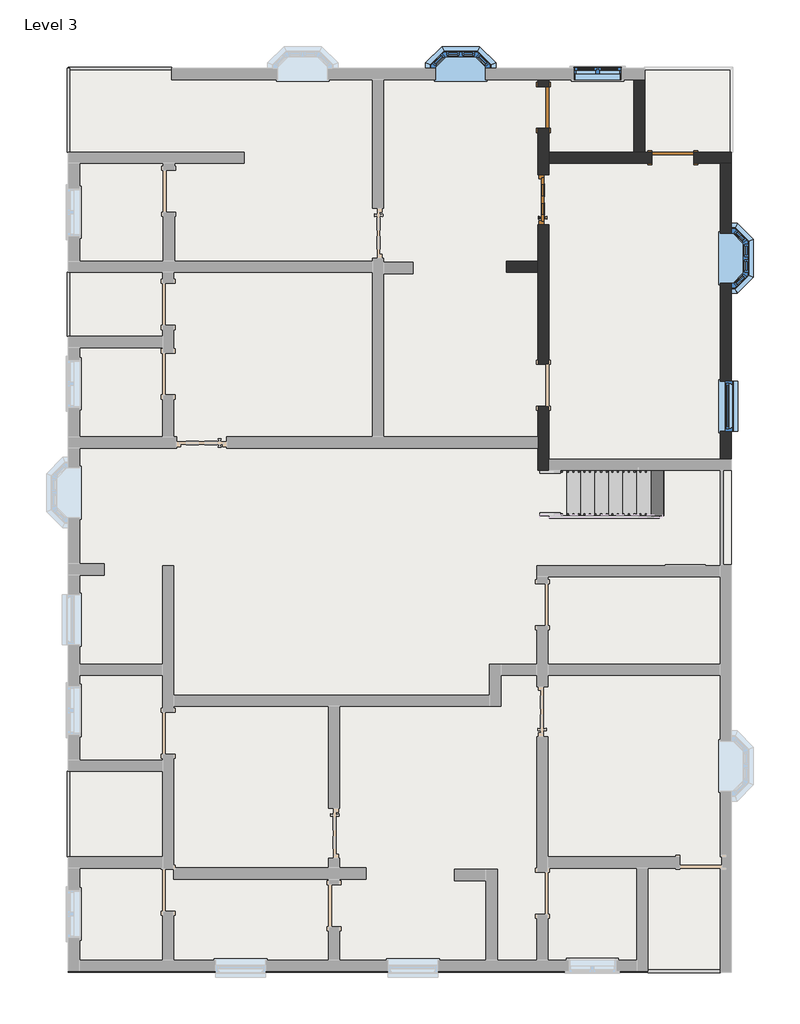
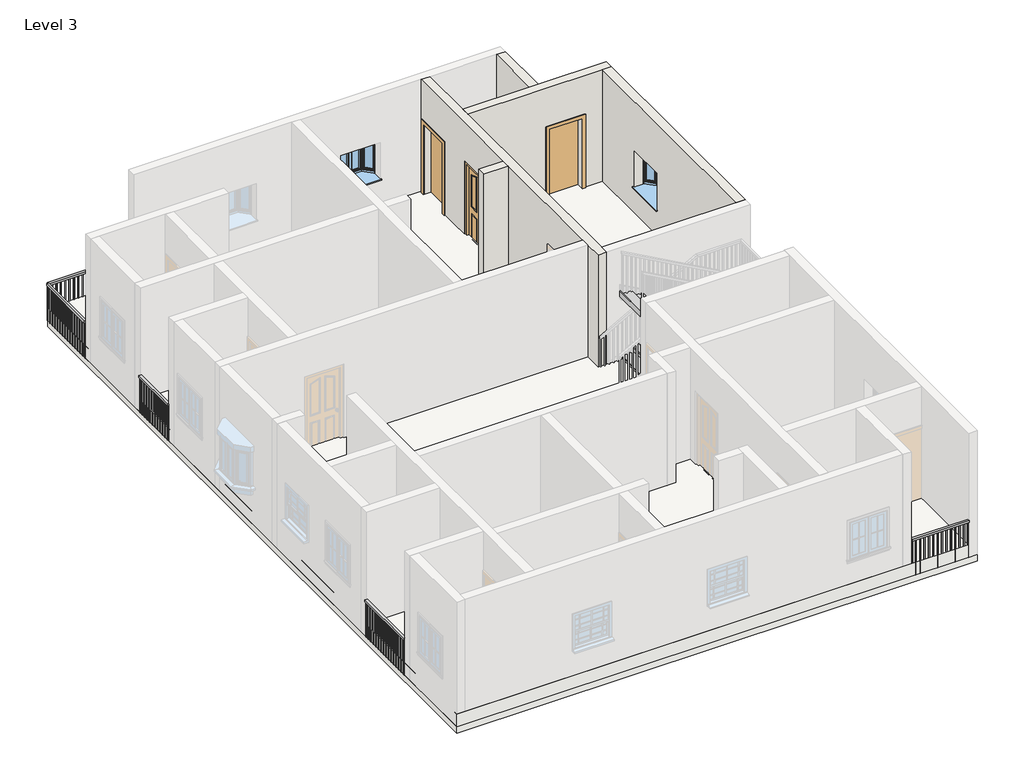
# One storey, part 2 of 4: 5 railings, 5 walls, 4 windows, 3 doors, 1 roof, 1 slab, 1 stair flight.
"""IFC4 building model written with IfcOpenShell, lengths in millimetres."""

from ifc_helpers import new_model, si_unit, frame, origin, place, context, project, spatial, polyline, outline, extrude, faceted_brep, transform, mapped, element, save
from components import doors_extsgl_12_910x2110mm_9a09825e, door_53b1b562, stair_flight_3990532a, window_910x910mm_67ef725a, window_c29befe5, windows_sash_w_bars_1_910x910mm_b688f793

model = new_model("IFC4")

# Units and contexts
model_context = context("Model", 3, world=origin())
ifc_project = project(units=[si_unit("LENGTHUNIT", "METRE", prefix="MILLI")], contexts=[model_context])

# Site, building, storey
site = spatial("IfcSite", under=ifc_project)
building = spatial("IfcBuilding", under=site)
storey = spatial("IfcBuildingStorey", under=building, Name="Level 3", Elevation=6096.0)

# Doors
placement = place(None, origin())
doors_extsgl_12_910x2110mm_shape = doors_extsgl_12_910x2110mm_9a09825e(model_context)
element("IfcDoor", 1, ObjectType="Doors_ExtSgl_12 : 910x2110mm", at=placement, inside=storey, context=model_context, shape_type="MappedRepresentation", body=[
    mapped(doors_extsgl_12_910x2110mm_shape, transform((1600.6941283, 5934.0547293, 6096.0), x_axis=(0.0, 1.0, 0.0), y_axis=(-1.0, 0.0, 0.0), z_axis=(0.0, 0.0, 1.0))),
])
door_shape = door_53b1b562(model_context)
element("IfcDoor", 2, ObjectType="Single-Flush : 30\" x 80\"", at=placement, inside=storey, context=model_context, shape_type="MappedRepresentation", body=[
    mapped(door_shape, transform((1600.6941283, 7610.4547293, 6096.0), x_axis=(0.0, 1.0, 0.0), y_axis=(-1.0, 0.0, 0.0), z_axis=(0.0, 0.0, 1.0))),
])
element("IfcDoor", 3, ObjectType="Single-Flush : 30\" x 80\"", at=placement, inside=storey, context=model_context, shape_type="MappedRepresentation", body=[
    mapped(door_shape, transform((3962.8941283, 6696.0547293, 6096.0), x_axis=(-1.0, 0.0, 0.0), y_axis=(0.0, -1.0, 0.0), z_axis=(0.0, 0.0, 1.0))),
])

# Railings
element("IfcRailing", 4, ObjectType="Handrail - Rectangular", at=placement, inside=storey, context=model_context, shape_type="SweptSolid", body=[
    extrude(outline(polyline([(-7073.4058717, 4609.0339901), (-7022.6058717, 4609.0339901), (-7022.6058717, 3444.8547293), (-7073.4058717, 3444.8547293), (-7073.4058717, 4609.0339901)])), frame((0.0, 0.0, 6959.6), z_axis=(0.0, 0.0, 1.0), x_axis=(1.0, 0.0, 0.0)), (0.0, 0.0, 1.0), 50.8),
    extrude(outline(polyline([(-7057.5308717, 3500.9589901), (-7038.4808717, 3500.9589901), (-7038.4808717, 3481.9089901), (-7057.5308717, 3481.9089901), (-7057.5308717, 3500.9589901)])), frame((0.0, 0.0, 6096.0), z_axis=(0.0, 0.0, 1.0), x_axis=(1.0, 0.0, 0.0)), (0.0, 0.0, 1.0), 863.6),
    extrude(outline(polyline([(-7057.5308717, 3602.5589901), (-7038.4808717, 3602.5589901), (-7038.4808717, 3583.5089901), (-7057.5308717, 3583.5089901), (-7057.5308717, 3602.5589901)])), frame((0.0, 0.0, 6096.0), z_axis=(0.0, 0.0, 1.0), x_axis=(1.0, 0.0, 0.0)), (0.0, 0.0, 1.0), 863.6),
    extrude(outline(polyline([(-7057.5308717, 3704.1589901), (-7038.4808717, 3704.1589901), (-7038.4808717, 3685.1089901), (-7057.5308717, 3685.1089901), (-7057.5308717, 3704.1589901)])), frame((0.0, 0.0, 6096.0), z_axis=(0.0, 0.0, 1.0), x_axis=(1.0, 0.0, 0.0)), (0.0, 0.0, 1.0), 863.6),
    extrude(outline(polyline([(-7057.5308717, 3805.7589901), (-7038.4808717, 3805.7589901), (-7038.4808717, 3786.7089901), (-7057.5308717, 3786.7089901), (-7057.5308717, 3805.7589901)])), frame((0.0, 0.0, 6096.0), z_axis=(0.0, 0.0, 1.0), x_axis=(1.0, 0.0, 0.0)), (0.0, 0.0, 1.0), 863.6),
    extrude(outline(polyline([(-7057.5308717, 3907.3589901), (-7038.4808717, 3907.3589901), (-7038.4808717, 3888.3089901), (-7057.5308717, 3888.3089901), (-7057.5308717, 3907.3589901)])), frame((0.0, 0.0, 6096.0), z_axis=(0.0, 0.0, 1.0), x_axis=(1.0, 0.0, 0.0)), (0.0, 0.0, 1.0), 863.6),
    extrude(outline(polyline([(-7057.5308717, 4008.9589901), (-7038.4808717, 4008.9589901), (-7038.4808717, 3989.9089901), (-7057.5308717, 3989.9089901), (-7057.5308717, 4008.9589901)])), frame((0.0, 0.0, 6096.0), z_axis=(0.0, 0.0, 1.0), x_axis=(1.0, 0.0, 0.0)), (0.0, 0.0, 1.0), 863.6),
    extrude(outline(polyline([(-7057.5308717, 4110.5589901), (-7038.4808717, 4110.5589901), (-7038.4808717, 4091.5089901), (-7057.5308717, 4091.5089901), (-7057.5308717, 4110.5589901)])), frame((0.0, 0.0, 6096.0), z_axis=(0.0, 0.0, 1.0), x_axis=(1.0, 0.0, 0.0)), (0.0, 0.0, 1.0), 863.6),
    extrude(outline(polyline([(-7057.5308717, 4212.1589901), (-7038.4808717, 4212.1589901), (-7038.4808717, 4193.1089901), (-7057.5308717, 4193.1089901), (-7057.5308717, 4212.1589901)])), frame((0.0, 0.0, 6096.0), z_axis=(0.0, 0.0, 1.0), x_axis=(1.0, 0.0, 0.0)), (0.0, 0.0, 1.0), 863.6),
    extrude(outline(polyline([(-7057.5308717, 4313.7589901), (-7038.4808717, 4313.7589901), (-7038.4808717, 4294.7089901), (-7057.5308717, 4294.7089901), (-7057.5308717, 4313.7589901)])), frame((0.0, 0.0, 6096.0), z_axis=(0.0, 0.0, 1.0), x_axis=(1.0, 0.0, 0.0)), (0.0, 0.0, 1.0), 863.6),
    extrude(outline(polyline([(-7057.5308717, 4415.3589901), (-7038.4808717, 4415.3589901), (-7038.4808717, 4396.3089901), (-7057.5308717, 4396.3089901), (-7057.5308717, 4415.3589901)])), frame((0.0, 0.0, 6096.0), z_axis=(0.0, 0.0, 1.0), x_axis=(1.0, 0.0, 0.0)), (0.0, 0.0, 1.0), 863.6),
    extrude(outline(polyline([(-7057.5308717, 4516.9589901), (-7038.4808717, 4516.9589901), (-7038.4808717, 4497.9089901), (-7057.5308717, 4497.9089901), (-7057.5308717, 4516.9589901)])), frame((0.0, 0.0, 6096.0), z_axis=(0.0, 0.0, 1.0), x_axis=(1.0, 0.0, 0.0)), (0.0, 0.0, 1.0), 863.6),
    extrude(outline(polyline([(-7057.5308717, 3463.9047293), (-7038.4808717, 3463.9047293), (-7038.4808717, 3444.8547293), (-7057.5308717, 3444.8547293), (-7057.5308717, 3463.9047293)])), frame((0.0, 0.0, 6096.0), z_axis=(0.0, 0.0, 1.0), x_axis=(1.0, 0.0, 0.0)), (0.0, 0.0, 1.0), 863.6),
    extrude(outline(polyline([(-7057.5308717, 4609.0339901), (-7038.4808717, 4609.0339901), (-7038.4808717, 4589.9839901), (-7057.5308717, 4589.9839901), (-7057.5308717, 4609.0339901)])), frame((0.0, 0.0, 6096.0), z_axis=(0.0, 0.0, 1.0), x_axis=(1.0, 0.0, 0.0)), (0.0, 0.0, 1.0), 863.6),
])
element("IfcRailing", 5, ObjectType="Handrail - Rectangular", at=placement, inside=storey, context=model_context, shape_type="SweptSolid", body=[
    extrude(outline(polyline([(-7073.4058717, -4474.6886333), (-7022.6058717, -4474.6886333), (-7022.6058717, -6029.3452707), (-7073.4058717, -6029.3452707), (-7073.4058717, -4474.6886333)])), frame((0.0, 0.0, 6959.6), z_axis=(0.0, 0.0, 1.0), x_axis=(1.0, 0.0, 0.0)), (0.0, 0.0, 1.0), 50.8),
    extrude(outline(polyline([(-7057.5308717, -5989.1636333), (-7038.4808717, -5989.1636333), (-7038.4808717, -6008.2136333), (-7057.5308717, -6008.2136333), (-7057.5308717, -5989.1636333)])), frame((0.0, 0.0, 6096.0), z_axis=(0.0, 0.0, 1.0), x_axis=(1.0, 0.0, 0.0)), (0.0, 0.0, 1.0), 863.6),
    extrude(outline(polyline([(-7057.5308717, -5887.5636333), (-7038.4808717, -5887.5636333), (-7038.4808717, -5906.6136333), (-7057.5308717, -5906.6136333), (-7057.5308717, -5887.5636333)])), frame((0.0, 0.0, 6096.0), z_axis=(0.0, 0.0, 1.0), x_axis=(1.0, 0.0, 0.0)), (0.0, 0.0, 1.0), 863.6),
    extrude(outline(polyline([(-7057.5308717, -5785.9636333), (-7038.4808717, -5785.9636333), (-7038.4808717, -5805.0136333), (-7057.5308717, -5805.0136333), (-7057.5308717, -5785.9636333)])), frame((0.0, 0.0, 6096.0), z_axis=(0.0, 0.0, 1.0), x_axis=(1.0, 0.0, 0.0)), (0.0, 0.0, 1.0), 863.6),
    extrude(outline(polyline([(-7057.5308717, -5684.3636333), (-7038.4808717, -5684.3636333), (-7038.4808717, -5703.4136333), (-7057.5308717, -5703.4136333), (-7057.5308717, -5684.3636333)])), frame((0.0, 0.0, 6096.0), z_axis=(0.0, 0.0, 1.0), x_axis=(1.0, 0.0, 0.0)), (0.0, 0.0, 1.0), 863.6),
    extrude(outline(polyline([(-7057.5308717, -5582.7636333), (-7038.4808717, -5582.7636333), (-7038.4808717, -5601.8136333), (-7057.5308717, -5601.8136333), (-7057.5308717, -5582.7636333)])), frame((0.0, 0.0, 6096.0), z_axis=(0.0, 0.0, 1.0), x_axis=(1.0, 0.0, 0.0)), (0.0, 0.0, 1.0), 863.6),
    extrude(outline(polyline([(-7057.5308717, -5481.1636333), (-7038.4808717, -5481.1636333), (-7038.4808717, -5500.2136333), (-7057.5308717, -5500.2136333), (-7057.5308717, -5481.1636333)])), frame((0.0, 0.0, 6096.0), z_axis=(0.0, 0.0, 1.0), x_axis=(1.0, 0.0, 0.0)), (0.0, 0.0, 1.0), 863.6),
    extrude(outline(polyline([(-7057.5308717, -5379.5636333), (-7038.4808717, -5379.5636333), (-7038.4808717, -5398.6136333), (-7057.5308717, -5398.6136333), (-7057.5308717, -5379.5636333)])), frame((0.0, 0.0, 6096.0), z_axis=(0.0, 0.0, 1.0), x_axis=(1.0, 0.0, 0.0)), (0.0, 0.0, 1.0), 863.6),
    extrude(outline(polyline([(-7057.5308717, -5277.9636333), (-7038.4808717, -5277.9636333), (-7038.4808717, -5297.0136333), (-7057.5308717, -5297.0136333), (-7057.5308717, -5277.9636333)])), frame((0.0, 0.0, 6096.0), z_axis=(0.0, 0.0, 1.0), x_axis=(1.0, 0.0, 0.0)), (0.0, 0.0, 1.0), 863.6),
    extrude(outline(polyline([(-7057.5308717, -5176.3636333), (-7038.4808717, -5176.3636333), (-7038.4808717, -5195.4136333), (-7057.5308717, -5195.4136333), (-7057.5308717, -5176.3636333)])), frame((0.0, 0.0, 6096.0), z_axis=(0.0, 0.0, 1.0), x_axis=(1.0, 0.0, 0.0)), (0.0, 0.0, 1.0), 863.6),
    extrude(outline(polyline([(-7057.5308717, -5074.7636333), (-7038.4808717, -5074.7636333), (-7038.4808717, -5093.8136333), (-7057.5308717, -5093.8136333), (-7057.5308717, -5074.7636333)])), frame((0.0, 0.0, 6096.0), z_axis=(0.0, 0.0, 1.0), x_axis=(1.0, 0.0, 0.0)), (0.0, 0.0, 1.0), 863.6),
    extrude(outline(polyline([(-7057.5308717, -4973.1636333), (-7038.4808717, -4973.1636333), (-7038.4808717, -4992.2136333), (-7057.5308717, -4992.2136333), (-7057.5308717, -4973.1636333)])), frame((0.0, 0.0, 6096.0), z_axis=(0.0, 0.0, 1.0), x_axis=(1.0, 0.0, 0.0)), (0.0, 0.0, 1.0), 863.6),
    extrude(outline(polyline([(-7057.5308717, -4871.5636333), (-7038.4808717, -4871.5636333), (-7038.4808717, -4890.6136333), (-7057.5308717, -4890.6136333), (-7057.5308717, -4871.5636333)])), frame((0.0, 0.0, 6096.0), z_axis=(0.0, 0.0, 1.0), x_axis=(1.0, 0.0, 0.0)), (0.0, 0.0, 1.0), 863.6),
    extrude(outline(polyline([(-7057.5308717, -4769.9636333), (-7038.4808717, -4769.9636333), (-7038.4808717, -4789.0136333), (-7057.5308717, -4789.0136333), (-7057.5308717, -4769.9636333)])), frame((0.0, 0.0, 6096.0), z_axis=(0.0, 0.0, 1.0), x_axis=(1.0, 0.0, 0.0)), (0.0, 0.0, 1.0), 863.6),
    extrude(outline(polyline([(-7057.5308717, -4668.3636333), (-7038.4808717, -4668.3636333), (-7038.4808717, -4687.4136333), (-7057.5308717, -4687.4136333), (-7057.5308717, -4668.3636333)])), frame((0.0, 0.0, 6096.0), z_axis=(0.0, 0.0, 1.0), x_axis=(1.0, 0.0, 0.0)), (0.0, 0.0, 1.0), 863.6),
    extrude(outline(polyline([(-7057.5308717, -4566.7636333), (-7038.4808717, -4566.7636333), (-7038.4808717, -4585.8136333), (-7057.5308717, -4585.8136333), (-7057.5308717, -4566.7636333)])), frame((0.0, 0.0, 6096.0), z_axis=(0.0, 0.0, 1.0), x_axis=(1.0, 0.0, 0.0)), (0.0, 0.0, 1.0), 863.6),
    extrude(outline(polyline([(-7057.5308717, -6010.2952707), (-7038.4808717, -6010.2952707), (-7038.4808717, -6029.3452707), (-7057.5308717, -6029.3452707), (-7057.5308717, -6010.2952707)])), frame((0.0, 0.0, 6096.0), z_axis=(0.0, 0.0, 1.0), x_axis=(1.0, 0.0, 0.0)), (0.0, 0.0, 1.0), 863.6),
    extrude(outline(polyline([(-7057.5308717, -4474.6886333), (-7038.4808717, -4474.6886333), (-7038.4808717, -4493.7386333), (-7057.5308717, -4493.7386333), (-7057.5308717, -4474.6886333)])), frame((0.0, 0.0, 6096.0), z_axis=(0.0, 0.0, 1.0), x_axis=(1.0, 0.0, 0.0)), (0.0, 0.0, 1.0), 863.6),
])
element("IfcRailing", 6, ObjectType="Handrail - Rectangular", at=placement, inside=storey, context=model_context, shape_type="SweptSolid", body=[
    extrude(outline(polyline([(3505.6941283, -8137.5452707), (3505.6941283, -8086.7452707), (4826.4941283, -8086.7452707), (4826.4941283, -8137.5452707), (3505.6941283, -8137.5452707)])), frame((0.0, 0.0, 6959.6), z_axis=(0.0, 0.0, 1.0), x_axis=(1.0, 0.0, 0.0)), (0.0, 0.0, 1.0), 50.8),
    extrude(outline(polyline([(4715.3691283, -8121.6702707), (4715.3691283, -8102.6202707), (4734.4191283, -8102.6202707), (4734.4191283, -8121.6702707), (4715.3691283, -8121.6702707)])), frame((0.0, 0.0, 6096.0), z_axis=(0.0, 0.0, 1.0), x_axis=(1.0, 0.0, 0.0)), (0.0, 0.0, 1.0), 863.6),
    extrude(outline(polyline([(4613.7691283, -8121.6702707), (4613.7691283, -8102.6202707), (4632.8191283, -8102.6202707), (4632.8191283, -8121.6702707), (4613.7691283, -8121.6702707)])), frame((0.0, 0.0, 6096.0), z_axis=(0.0, 0.0, 1.0), x_axis=(1.0, 0.0, 0.0)), (0.0, 0.0, 1.0), 863.6),
    extrude(outline(polyline([(4512.1691283, -8121.6702707), (4512.1691283, -8102.6202707), (4531.2191283, -8102.6202707), (4531.2191283, -8121.6702707), (4512.1691283, -8121.6702707)])), frame((0.0, 0.0, 6096.0), z_axis=(0.0, 0.0, 1.0), x_axis=(1.0, 0.0, 0.0)), (0.0, 0.0, 1.0), 863.6),
    extrude(outline(polyline([(4410.5691283, -8121.6702707), (4410.5691283, -8102.6202707), (4429.6191283, -8102.6202707), (4429.6191283, -8121.6702707), (4410.5691283, -8121.6702707)])), frame((0.0, 0.0, 6096.0), z_axis=(0.0, 0.0, 1.0), x_axis=(1.0, 0.0, 0.0)), (0.0, 0.0, 1.0), 863.6),
    extrude(outline(polyline([(4308.9691283, -8121.6702707), (4308.9691283, -8102.6202707), (4328.0191283, -8102.6202707), (4328.0191283, -8121.6702707), (4308.9691283, -8121.6702707)])), frame((0.0, 0.0, 6096.0), z_axis=(0.0, 0.0, 1.0), x_axis=(1.0, 0.0, 0.0)), (0.0, 0.0, 1.0), 863.6),
    extrude(outline(polyline([(4207.3691283, -8121.6702707), (4207.3691283, -8102.6202707), (4226.4191283, -8102.6202707), (4226.4191283, -8121.6702707), (4207.3691283, -8121.6702707)])), frame((0.0, 0.0, 6096.0), z_axis=(0.0, 0.0, 1.0), x_axis=(1.0, 0.0, 0.0)), (0.0, 0.0, 1.0), 863.6),
    extrude(outline(polyline([(4105.7691283, -8121.6702707), (4105.7691283, -8102.6202707), (4124.8191283, -8102.6202707), (4124.8191283, -8121.6702707), (4105.7691283, -8121.6702707)])), frame((0.0, 0.0, 6096.0), z_axis=(0.0, 0.0, 1.0), x_axis=(1.0, 0.0, 0.0)), (0.0, 0.0, 1.0), 863.6),
    extrude(outline(polyline([(4004.1691283, -8121.6702707), (4004.1691283, -8102.6202707), (4023.2191283, -8102.6202707), (4023.2191283, -8121.6702707), (4004.1691283, -8121.6702707)])), frame((0.0, 0.0, 6096.0), z_axis=(0.0, 0.0, 1.0), x_axis=(1.0, 0.0, 0.0)), (0.0, 0.0, 1.0), 863.6),
    extrude(outline(polyline([(3902.5691283, -8121.6702707), (3902.5691283, -8102.6202707), (3921.6191283, -8102.6202707), (3921.6191283, -8121.6702707), (3902.5691283, -8121.6702707)])), frame((0.0, 0.0, 6096.0), z_axis=(0.0, 0.0, 1.0), x_axis=(1.0, 0.0, 0.0)), (0.0, 0.0, 1.0), 863.6),
    extrude(outline(polyline([(3800.9691283, -8121.6702707), (3800.9691283, -8102.6202707), (3820.0191283, -8102.6202707), (3820.0191283, -8121.6702707), (3800.9691283, -8121.6702707)])), frame((0.0, 0.0, 6096.0), z_axis=(0.0, 0.0, 1.0), x_axis=(1.0, 0.0, 0.0)), (0.0, 0.0, 1.0), 863.6),
    extrude(outline(polyline([(3699.3691283, -8121.6702707), (3699.3691283, -8102.6202707), (3718.4191283, -8102.6202707), (3718.4191283, -8121.6702707), (3699.3691283, -8121.6702707)])), frame((0.0, 0.0, 6096.0), z_axis=(0.0, 0.0, 1.0), x_axis=(1.0, 0.0, 0.0)), (0.0, 0.0, 1.0), 863.6),
    extrude(outline(polyline([(3597.7691283, -8121.6702707), (3597.7691283, -8102.6202707), (3616.8191283, -8102.6202707), (3616.8191283, -8121.6702707), (3597.7691283, -8121.6702707)])), frame((0.0, 0.0, 6096.0), z_axis=(0.0, 0.0, 1.0), x_axis=(1.0, 0.0, 0.0)), (0.0, 0.0, 1.0), 863.6),
    extrude(outline(polyline([(4807.4441283, -8121.6702707), (4807.4441283, -8102.6202707), (4826.4941283, -8102.6202707), (4826.4941283, -8121.6702707), (4807.4441283, -8121.6702707)])), frame((0.0, 0.0, 6096.0), z_axis=(0.0, 0.0, 1.0), x_axis=(1.0, 0.0, 0.0)), (0.0, 0.0, 1.0), 863.6),
    extrude(outline(polyline([(3505.6941283, -8121.6702707), (3505.6941283, -8102.6202707), (3524.7441283, -8102.6202707), (3524.7441283, -8121.6702707), (3505.6941283, -8121.6702707)])), frame((0.0, 0.0, 6096.0), z_axis=(0.0, 0.0, 1.0), x_axis=(1.0, 0.0, 0.0)), (0.0, 0.0, 1.0), 863.6),
])
element("IfcRailing", 7, ObjectType="Handrail - Rectangular", at=placement, inside=storey, context=model_context, shape_type="SweptSolid", body=[
    extrude(outline(polyline([(-7022.6058717, 6797.6547293), (-7073.4058717, 6797.6547293), (-7073.4058717, 8321.6547293), (-7022.6058717, 8321.6547293), (-7022.6058717, 6797.6547293)])), frame((0.0, 0.0, 6959.6), z_axis=(0.0, 0.0, 1.0), x_axis=(1.0, 0.0, 0.0)), (0.0, 0.0, 1.0), 50.8),
    extrude(outline(polyline([(-7038.4808717, 8210.5297293), (-7057.5308717, 8210.5297293), (-7057.5308717, 8229.5797293), (-7038.4808717, 8229.5797293), (-7038.4808717, 8210.5297293)])), frame((0.0, 0.0, 6096.0), z_axis=(0.0, 0.0, 1.0), x_axis=(1.0, 0.0, 0.0)), (0.0, 0.0, 1.0), 863.6),
    extrude(outline(polyline([(-7038.4808717, 8108.9297293), (-7057.5308717, 8108.9297293), (-7057.5308717, 8127.9797293), (-7038.4808717, 8127.9797293), (-7038.4808717, 8108.9297293)])), frame((0.0, 0.0, 6096.0), z_axis=(0.0, 0.0, 1.0), x_axis=(1.0, 0.0, 0.0)), (0.0, 0.0, 1.0), 863.6),
    extrude(outline(polyline([(-7038.4808717, 8007.3297293), (-7057.5308717, 8007.3297293), (-7057.5308717, 8026.3797293), (-7038.4808717, 8026.3797293), (-7038.4808717, 8007.3297293)])), frame((0.0, 0.0, 6096.0), z_axis=(0.0, 0.0, 1.0), x_axis=(1.0, 0.0, 0.0)), (0.0, 0.0, 1.0), 863.6),
    extrude(outline(polyline([(-7038.4808717, 7905.7297293), (-7057.5308717, 7905.7297293), (-7057.5308717, 7924.7797293), (-7038.4808717, 7924.7797293), (-7038.4808717, 7905.7297293)])), frame((0.0, 0.0, 6096.0), z_axis=(0.0, 0.0, 1.0), x_axis=(1.0, 0.0, 0.0)), (0.0, 0.0, 1.0), 863.6),
    extrude(outline(polyline([(-7038.4808717, 7804.1297293), (-7057.5308717, 7804.1297293), (-7057.5308717, 7823.1797293), (-7038.4808717, 7823.1797293), (-7038.4808717, 7804.1297293)])), frame((0.0, 0.0, 6096.0), z_axis=(0.0, 0.0, 1.0), x_axis=(1.0, 0.0, 0.0)), (0.0, 0.0, 1.0), 863.6),
    extrude(outline(polyline([(-7038.4808717, 7702.5297293), (-7057.5308717, 7702.5297293), (-7057.5308717, 7721.5797293), (-7038.4808717, 7721.5797293), (-7038.4808717, 7702.5297293)])), frame((0.0, 0.0, 6096.0), z_axis=(0.0, 0.0, 1.0), x_axis=(1.0, 0.0, 0.0)), (0.0, 0.0, 1.0), 863.6),
    extrude(outline(polyline([(-7038.4808717, 7600.9297293), (-7057.5308717, 7600.9297293), (-7057.5308717, 7619.9797293), (-7038.4808717, 7619.9797293), (-7038.4808717, 7600.9297293)])), frame((0.0, 0.0, 6096.0), z_axis=(0.0, 0.0, 1.0), x_axis=(1.0, 0.0, 0.0)), (0.0, 0.0, 1.0), 863.6),
    extrude(outline(polyline([(-7038.4808717, 7499.3297293), (-7057.5308717, 7499.3297293), (-7057.5308717, 7518.3797293), (-7038.4808717, 7518.3797293), (-7038.4808717, 7499.3297293)])), frame((0.0, 0.0, 6096.0), z_axis=(0.0, 0.0, 1.0), x_axis=(1.0, 0.0, 0.0)), (0.0, 0.0, 1.0), 863.6),
    extrude(outline(polyline([(-7038.4808717, 7397.7297293), (-7057.5308717, 7397.7297293), (-7057.5308717, 7416.7797293), (-7038.4808717, 7416.7797293), (-7038.4808717, 7397.7297293)])), frame((0.0, 0.0, 6096.0), z_axis=(0.0, 0.0, 1.0), x_axis=(1.0, 0.0, 0.0)), (0.0, 0.0, 1.0), 863.6),
    extrude(outline(polyline([(-7038.4808717, 7296.1297293), (-7057.5308717, 7296.1297293), (-7057.5308717, 7315.1797293), (-7038.4808717, 7315.1797293), (-7038.4808717, 7296.1297293)])), frame((0.0, 0.0, 6096.0), z_axis=(0.0, 0.0, 1.0), x_axis=(1.0, 0.0, 0.0)), (0.0, 0.0, 1.0), 863.6),
    extrude(outline(polyline([(-7038.4808717, 7194.5297293), (-7057.5308717, 7194.5297293), (-7057.5308717, 7213.5797293), (-7038.4808717, 7213.5797293), (-7038.4808717, 7194.5297293)])), frame((0.0, 0.0, 6096.0), z_axis=(0.0, 0.0, 1.0), x_axis=(1.0, 0.0, 0.0)), (0.0, 0.0, 1.0), 863.6),
    extrude(outline(polyline([(-7038.4808717, 7092.9297293), (-7057.5308717, 7092.9297293), (-7057.5308717, 7111.9797293), (-7038.4808717, 7111.9797293), (-7038.4808717, 7092.9297293)])), frame((0.0, 0.0, 6096.0), z_axis=(0.0, 0.0, 1.0), x_axis=(1.0, 0.0, 0.0)), (0.0, 0.0, 1.0), 863.6),
    extrude(outline(polyline([(-7038.4808717, 6991.3297293), (-7057.5308717, 6991.3297293), (-7057.5308717, 7010.3797293), (-7038.4808717, 7010.3797293), (-7038.4808717, 6991.3297293)])), frame((0.0, 0.0, 6096.0), z_axis=(0.0, 0.0, 1.0), x_axis=(1.0, 0.0, 0.0)), (0.0, 0.0, 1.0), 863.6),
    extrude(outline(polyline([(-7038.4808717, 6889.7297293), (-7057.5308717, 6889.7297293), (-7057.5308717, 6908.7797293), (-7038.4808717, 6908.7797293), (-7038.4808717, 6889.7297293)])), frame((0.0, 0.0, 6096.0), z_axis=(0.0, 0.0, 1.0), x_axis=(1.0, 0.0, 0.0)), (0.0, 0.0, 1.0), 863.6),
    extrude(outline(polyline([(-7038.4808717, 8302.6047293), (-7057.5308717, 8302.6047293), (-7057.5308717, 8321.6547293), (-7038.4808717, 8321.6547293), (-7038.4808717, 8302.6047293)])), frame((0.0, 0.0, 6096.0), z_axis=(0.0, 0.0, 1.0), x_axis=(1.0, 0.0, 0.0)), (0.0, 0.0, 1.0), 863.6),
    extrude(outline(polyline([(-7038.4808717, 6797.6547293), (-7057.5308717, 6797.6547293), (-7057.5308717, 6816.7047293), (-7038.4808717, 6816.7047293), (-7038.4808717, 6797.6547293)])), frame((0.0, 0.0, 6096.0), z_axis=(0.0, 0.0, 1.0), x_axis=(1.0, 0.0, 0.0)), (0.0, 0.0, 1.0), 863.6),
])
element("IfcRailing", 8, ObjectType="Handrail - Rectangular", at=placement, inside=storey, context=model_context, shape_type="SweptSolid", body=[
    extrude(outline(polyline([(-7048.0058717, 8296.2547293), (-7048.0058717, 8347.0547293), (-5168.4058717, 8347.0547293), (-5168.4058717, 8296.2547293), (-7048.0058717, 8296.2547293)])), frame((0.0, 0.0, 6959.6), z_axis=(0.0, 0.0, 1.0), x_axis=(1.0, 0.0, 0.0)), (0.0, 0.0, 1.0), 50.8),
    extrude(outline(polyline([(-5228.7308717, 8312.1297293), (-5228.7308717, 8331.1797293), (-5209.6808717, 8331.1797293), (-5209.6808717, 8312.1297293), (-5228.7308717, 8312.1297293)])), frame((0.0, 0.0, 6096.0), z_axis=(0.0, 0.0, 1.0), x_axis=(1.0, 0.0, 0.0)), (0.0, 0.0, 1.0), 863.6),
    extrude(outline(polyline([(-5330.3308717, 8312.1297293), (-5330.3308717, 8331.1797293), (-5311.2808717, 8331.1797293), (-5311.2808717, 8312.1297293), (-5330.3308717, 8312.1297293)])), frame((0.0, 0.0, 6096.0), z_axis=(0.0, 0.0, 1.0), x_axis=(1.0, 0.0, 0.0)), (0.0, 0.0, 1.0), 863.6),
    extrude(outline(polyline([(-5431.9308717, 8312.1297293), (-5431.9308717, 8331.1797293), (-5412.8808717, 8331.1797293), (-5412.8808717, 8312.1297293), (-5431.9308717, 8312.1297293)])), frame((0.0, 0.0, 6096.0), z_axis=(0.0, 0.0, 1.0), x_axis=(1.0, 0.0, 0.0)), (0.0, 0.0, 1.0), 863.6),
    extrude(outline(polyline([(-5533.5308717, 8312.1297293), (-5533.5308717, 8331.1797293), (-5514.4808717, 8331.1797293), (-5514.4808717, 8312.1297293), (-5533.5308717, 8312.1297293)])), frame((0.0, 0.0, 6096.0), z_axis=(0.0, 0.0, 1.0), x_axis=(1.0, 0.0, 0.0)), (0.0, 0.0, 1.0), 863.6),
    extrude(outline(polyline([(-5635.1308717, 8312.1297293), (-5635.1308717, 8331.1797293), (-5616.0808717, 8331.1797293), (-5616.0808717, 8312.1297293), (-5635.1308717, 8312.1297293)])), frame((0.0, 0.0, 6096.0), z_axis=(0.0, 0.0, 1.0), x_axis=(1.0, 0.0, 0.0)), (0.0, 0.0, 1.0), 863.6),
    extrude(outline(polyline([(-5736.7308717, 8312.1297293), (-5736.7308717, 8331.1797293), (-5717.6808717, 8331.1797293), (-5717.6808717, 8312.1297293), (-5736.7308717, 8312.1297293)])), frame((0.0, 0.0, 6096.0), z_axis=(0.0, 0.0, 1.0), x_axis=(1.0, 0.0, 0.0)), (0.0, 0.0, 1.0), 863.6),
    extrude(outline(polyline([(-5838.3308717, 8312.1297293), (-5838.3308717, 8331.1797293), (-5819.2808717, 8331.1797293), (-5819.2808717, 8312.1297293), (-5838.3308717, 8312.1297293)])), frame((0.0, 0.0, 6096.0), z_axis=(0.0, 0.0, 1.0), x_axis=(1.0, 0.0, 0.0)), (0.0, 0.0, 1.0), 863.6),
    extrude(outline(polyline([(-5939.9308717, 8312.1297293), (-5939.9308717, 8331.1797293), (-5920.8808717, 8331.1797293), (-5920.8808717, 8312.1297293), (-5939.9308717, 8312.1297293)])), frame((0.0, 0.0, 6096.0), z_axis=(0.0, 0.0, 1.0), x_axis=(1.0, 0.0, 0.0)), (0.0, 0.0, 1.0), 863.6),
    extrude(outline(polyline([(-6041.5308717, 8312.1297293), (-6041.5308717, 8331.1797293), (-6022.4808717, 8331.1797293), (-6022.4808717, 8312.1297293), (-6041.5308717, 8312.1297293)])), frame((0.0, 0.0, 6096.0), z_axis=(0.0, 0.0, 1.0), x_axis=(1.0, 0.0, 0.0)), (0.0, 0.0, 1.0), 863.6),
    extrude(outline(polyline([(-6143.1308717, 8312.1297293), (-6143.1308717, 8331.1797293), (-6124.0808717, 8331.1797293), (-6124.0808717, 8312.1297293), (-6143.1308717, 8312.1297293)])), frame((0.0, 0.0, 6096.0), z_axis=(0.0, 0.0, 1.0), x_axis=(1.0, 0.0, 0.0)), (0.0, 0.0, 1.0), 863.6),
    extrude(outline(polyline([(-6244.7308717, 8312.1297293), (-6244.7308717, 8331.1797293), (-6225.6808717, 8331.1797293), (-6225.6808717, 8312.1297293), (-6244.7308717, 8312.1297293)])), frame((0.0, 0.0, 6096.0), z_axis=(0.0, 0.0, 1.0), x_axis=(1.0, 0.0, 0.0)), (0.0, 0.0, 1.0), 863.6),
    extrude(outline(polyline([(-6346.3308717, 8312.1297293), (-6346.3308717, 8331.1797293), (-6327.2808717, 8331.1797293), (-6327.2808717, 8312.1297293), (-6346.3308717, 8312.1297293)])), frame((0.0, 0.0, 6096.0), z_axis=(0.0, 0.0, 1.0), x_axis=(1.0, 0.0, 0.0)), (0.0, 0.0, 1.0), 863.6),
    extrude(outline(polyline([(-6447.9308717, 8312.1297293), (-6447.9308717, 8331.1797293), (-6428.8808717, 8331.1797293), (-6428.8808717, 8312.1297293), (-6447.9308717, 8312.1297293)])), frame((0.0, 0.0, 6096.0), z_axis=(0.0, 0.0, 1.0), x_axis=(1.0, 0.0, 0.0)), (0.0, 0.0, 1.0), 863.6),
    extrude(outline(polyline([(-6549.5308717, 8312.1297293), (-6549.5308717, 8331.1797293), (-6530.4808717, 8331.1797293), (-6530.4808717, 8312.1297293), (-6549.5308717, 8312.1297293)])), frame((0.0, 0.0, 6096.0), z_axis=(0.0, 0.0, 1.0), x_axis=(1.0, 0.0, 0.0)), (0.0, 0.0, 1.0), 863.6),
    extrude(outline(polyline([(-6651.1308717, 8312.1297293), (-6651.1308717, 8331.1797293), (-6632.0808717, 8331.1797293), (-6632.0808717, 8312.1297293), (-6651.1308717, 8312.1297293)])), frame((0.0, 0.0, 6096.0), z_axis=(0.0, 0.0, 1.0), x_axis=(1.0, 0.0, 0.0)), (0.0, 0.0, 1.0), 863.6),
    extrude(outline(polyline([(-6752.7308717, 8312.1297293), (-6752.7308717, 8331.1797293), (-6733.6808717, 8331.1797293), (-6733.6808717, 8312.1297293), (-6752.7308717, 8312.1297293)])), frame((0.0, 0.0, 6096.0), z_axis=(0.0, 0.0, 1.0), x_axis=(1.0, 0.0, 0.0)), (0.0, 0.0, 1.0), 863.6),
    extrude(outline(polyline([(-6854.3308717, 8312.1297293), (-6854.3308717, 8331.1797293), (-6835.2808717, 8331.1797293), (-6835.2808717, 8312.1297293), (-6854.3308717, 8312.1297293)])), frame((0.0, 0.0, 6096.0), z_axis=(0.0, 0.0, 1.0), x_axis=(1.0, 0.0, 0.0)), (0.0, 0.0, 1.0), 863.6),
    extrude(outline(polyline([(-6955.9308717, 8312.1297293), (-6955.9308717, 8331.1797293), (-6936.8808717, 8331.1797293), (-6936.8808717, 8312.1297293), (-6955.9308717, 8312.1297293)])), frame((0.0, 0.0, 6096.0), z_axis=(0.0, 0.0, 1.0), x_axis=(1.0, 0.0, 0.0)), (0.0, 0.0, 1.0), 863.6),
    extrude(outline(polyline([(-5187.4558717, 8312.1297293), (-5187.4558717, 8331.1797293), (-5168.4058717, 8331.1797293), (-5168.4058717, 8312.1297293), (-5187.4558717, 8312.1297293)])), frame((0.0, 0.0, 6096.0), z_axis=(0.0, 0.0, 1.0), x_axis=(1.0, 0.0, 0.0)), (0.0, 0.0, 1.0), 863.6),
    extrude(outline(polyline([(-7048.0058717, 8312.1297293), (-7048.0058717, 8331.1797293), (-7028.9558717, 8331.1797293), (-7028.9558717, 8312.1297293), (-7048.0058717, 8312.1297293)])), frame((0.0, 0.0, 6096.0), z_axis=(0.0, 0.0, 1.0), x_axis=(1.0, 0.0, 0.0)), (0.0, 0.0, 1.0), 863.6),
])

# Roof
element("IfcRoof", 9, ObjectType="Generic - 12\"", at=placement, inside=storey, context=model_context, shape_type="SweptSolid", body=[
    extrude(outline(polyline([(-7048.0058717, 8321.6547293), (5029.6941283, 8321.6547293), (5029.6941283, -8124.8452707), (-7048.0058717, -8124.8452707), (-7048.0058717, 8321.6547293)])), frame((0.0, 0.0, 6096.0), z_axis=(0.0, 0.0, 1.0), x_axis=(1.0, 0.0, 0.0)), (0.0, 0.0, 1.0), 304.8),
])

# Slab
element("IfcSlab", 10, ObjectType="Generic - 12\"", at=placement, inside=storey, context=model_context, shape_type="SweptSolid", body=[
    extrude(outline(polyline([(5029.6941283, 8321.6547293), (5029.6941283, -8124.8452707), (-7048.0058717, -8124.8452707), (-7048.0058717, 8321.6547293), (5029.6941283, 8321.6547293)])), frame((0.0, 0.0, 5943.6), z_axis=(0.0, 0.0, 1.0), x_axis=(1.0, 0.0, 0.0)), (0.0, 0.0, 1.0), 152.4),
])

# Stair flight
stair_flight_shape = stair_flight_3990532a(model_context)
element("IfcStairFlight", 11, ObjectType="2\" Tread 1\" Nosing 1/4\" Riser", at=placement, inside=storey, context=model_context, shape_type="MappedRepresentation", body=[
    mapped(stair_flight_shape, transform((0.0, 0.0, 0.0), x_axis=(1.0, 0.0, 0.0), y_axis=(0.0, 1.0, 0.0), z_axis=(0.0, 0.0, 1.0))),
])

# Walls
element("IfcWall", 12, ObjectType="Generic - 4.5\"", at=placement, inside=storey, context=model_context, shape_type="Brep", body=[
    faceted_brep([(1499.0941283, 8118.4547293, 6096.0), (1499.0941283, 7991.4547293, 6096.0), (1499.0941283, 7991.4547293, 8128.0), (1499.0941283, 7229.4547293, 8128.0), (1499.0941283, 7229.4547293, 6096.0), (1499.0941283, 6389.0547293, 6096.0), (1499.0941283, 6389.0547293, 8206.0), (1499.0941283, 5479.0547293, 8206.0), (1499.0941283, 5479.0547293, 6096.0), (1499.0941283, 4812.2339901, 6096.0), (1499.0941283, 4609.0339901, 6096.0), (1499.0941283, 2936.8547293, 6096.0), (1499.0941283, 2936.8547293, 8128.0), (1499.0941283, 2174.8547293, 8128.0), (1499.0941283, 2174.8547293, 6096.0), (1499.0941283, 1616.0547293, 6096.0), (1499.0941283, 1412.8547293, 6096.0), (1499.0941283, 1006.4547293, 6096.0), (1499.0941283, 1006.4547293, 9144.0), (1499.0941283, 1412.8547293, 9144.0), (1499.0941283, 1616.0547293, 9144.0), (1499.0941283, 4609.0339901, 9144.0), (1499.0941283, 4812.2339901, 9144.0), (1499.0941283, 8118.4547293, 9144.0), (1702.2941283, 7991.4547293, 8128.0), (1702.2941283, 7991.4547293, 6096.0), (1702.2941283, 8118.4547293, 6096.0), (1702.2941283, 8118.4547293, 9144.0), (1702.2941283, 6797.6547293, 9144.0), (1702.2941283, 6594.4547293, 9144.0), (1702.2941283, 1209.6547293, 9144.0), (1702.2941283, 1006.4547293, 9144.0), (1702.2941283, 1006.4547293, 6096.0), (1702.2941283, 1209.6547293, 6096.0), (1702.2941283, 2174.8547293, 6096.0), (1702.2941283, 2174.8547293, 8128.0), (1702.2941283, 2936.8547293, 8128.0), (1702.2941283, 2936.8547293, 6096.0), (1702.2941283, 5479.0547293, 6096.0), (1702.2941283, 5479.0547293, 8206.0), (1702.2941283, 6389.0547293, 8206.0), (1702.2941283, 6389.0547293, 6096.0), (1702.2941283, 6594.4547293, 6096.0), (1702.2941283, 6797.6547293, 6096.0), (1702.2941283, 7229.4547293, 6096.0), (1702.2941283, 7229.4547293, 8128.0)], [[[0, 1, 2, 3, 4, 5, 6, 7, 8, 9, 10, 11, 12, 13, 14, 15, 16, 17, 18, 19, 20, 21, 22, 23]], [[24, 25, 26, 27, 28, 29, 30, 31, 32, 33, 34, 35, 36, 37, 38, 39, 40, 41, 42, 43, 44, 45]], [[38, 37, 11, 10, 9, 8]], [[34, 33, 32, 17, 16, 15, 14]], [[26, 25, 1, 0]], [[44, 43, 42, 41, 5, 4]], [[23, 22, 21, 20, 19, 18, 31, 30, 29, 28, 27]], [[0, 23, 27, 26]], [[18, 17, 32, 31]], [[8, 7, 39, 38]], [[6, 5, 41, 40]], [[7, 6, 40, 39]], [[12, 11, 37, 36]], [[13, 12, 36, 35]], [[14, 13, 35, 34]], [[2, 1, 25, 24]], [[3, 2, 24, 45]], [[4, 3, 45, 44]]]),
])
element("IfcWall", 13, ObjectType="Generic - 4.5\"", at=placement, inside=storey, context=model_context, shape_type="Brep", body=[
    faceted_brep([(1702.2941283, 6594.4547293, 6096.0), (3581.8941283, 6594.4547293, 6096.0), (3581.8941283, 6594.4547293, 8128.0), (4343.8941283, 6594.4547293, 8128.0), (4343.8941283, 6594.4547293, 6096.0), (4826.4941283, 6594.4547293, 6096.0), (5029.6941283, 6594.4547293, 6096.0), (5029.6941283, 6594.4547293, 9144.0), (4826.4941283, 6594.4547293, 9144.0), (1702.2941283, 6594.4547293, 9144.0), (3581.8941283, 6797.6547293, 8128.0), (3581.8941283, 6797.6547293, 6096.0), (3454.8941283, 6797.6547293, 6096.0), (3251.6941283, 6797.6547293, 6096.0), (1702.2941283, 6797.6547293, 6096.0), (1702.2941283, 6797.6547293, 9144.0), (3251.6941283, 6797.6547293, 9144.0), (3454.8941283, 6797.6547293, 9144.0), (5029.6941283, 6797.6547293, 9144.0), (5029.6941283, 6797.6547293, 6096.0), (4343.8941283, 6797.6547293, 6096.0), (4343.8941283, 6797.6547293, 8128.0)], [[[0, 1, 2, 3, 4, 5, 6, 7, 8, 9]], [[10, 11, 12, 13, 14, 15, 16, 17, 18, 19, 20, 21]], [[20, 19, 6, 5, 4]], [[14, 13, 12, 11, 1, 0]], [[9, 8, 7, 18, 17, 16, 15]], [[0, 9, 15, 14]], [[2, 1, 11, 10]], [[3, 2, 10, 21]], [[4, 3, 21, 20]], [[7, 6, 19, 18]]]),
])
element("IfcWall", 14, ObjectType="Generic - 4.5\"", at=placement, inside=storey, context=model_context, shape_type="SweptSolid", body=[
    extrude(outline(polyline([(3251.6941283, 6797.6547293), (3251.6941283, 8118.4547293), (3454.8941283, 8118.4547293), (3454.8941283, 6797.6547293), (3251.6941283, 6797.6547293)])), frame((0.0, 0.0, 6096.0), z_axis=(0.0, 0.0, 1.0), x_axis=(1.0, 0.0, 0.0)), (0.0, 0.0, 1.0), 3048.0),
])
element("IfcWall", 15, ObjectType="Generic - 4.5\"", at=placement, inside=storey, context=model_context, shape_type="SweptSolid", body=[
    extrude(outline(polyline([(927.5941283, 4812.2339901), (1499.0941283, 4812.2339901), (1499.0941283, 4609.0339901), (927.5941283, 4609.0339901), (927.5941283, 4812.2339901)])), frame((0.0, 0.0, 6096.0), z_axis=(0.0, 0.0, 1.0), x_axis=(1.0, 0.0, 0.0)), (0.0, 0.0, 1.0), 3048.0),
])
element("IfcWall", 16, ObjectType="Generic - 9\"", at=placement, inside=storey, context=model_context, shape_type="SweptSolid", body=[
    extrude(outline(polyline([(6594.4547293, 6096.0), (1209.6547293, 6096.0), (1209.6547293, 9144.0), (6594.4547293, 9144.0), (6594.4547293, 6096.0)]), holes=[polyline([(5322.2547293, 7920.4), (4412.2547293, 7920.4), (4412.2547293, 7010.4), (5322.2547293, 7010.4), (5322.2547293, 7920.4)]), polyline([(2629.8547293, 7010.4), (2629.8547293, 7920.4), (1719.8547293, 7920.4), (1719.8547293, 7010.4), (2629.8547293, 7010.4)])]), frame((4826.4941283, 0.0, 0.0), z_axis=(1.0, 0.0, 0.0), x_axis=(0.0, 1.0, 0.0)), (0.0, 0.0, 1.0), 203.2),
])

# Windows
window_910x910mm_shape = window_910x910mm_67ef725a(model_context)
element("IfcWindow", 17, ObjectType="910x910mm", at=placement, inside=storey, context=model_context, shape_type="MappedRepresentation", body=[
    mapped(window_910x910mm_shape, transform((4919.6375605, 4297.2547293, 5810.4), x_axis=(0.0, -1.0, 0.0), y_axis=(1.0, 0.0, 0.0), z_axis=(0.0, 0.0, 1.0))),
])
element("IfcWindow", 18, ObjectType="910x910mm", at=placement, inside=storey, context=model_context, shape_type="MappedRepresentation", body=[
    mapped(window_910x910mm_shape, transform((665.7441283, 8211.5981615, 5810.4), x_axis=(1.0, 0.0, 0.0), y_axis=(0.0, 1.0, 0.0), z_axis=(0.0, 0.0, 1.0))),
])
window_shape = window_c29befe5(model_context)
element("IfcWindow", 19, ObjectType="Window-Casement-Double : 34\" x 36\"", at=placement, inside=storey, context=model_context, shape_type="MappedRepresentation", body=[
    mapped(window_shape, transform((2591.2941283, 8220.0547293, 6096.0), x_axis=(1.0, 0.0, 0.0), y_axis=(0.0, 1.0, 0.0), z_axis=(0.0, 0.0, 1.0))),
])
windows_sash_w_bars_1_910x910mm_shape = windows_sash_w_bars_1_910x910mm_b688f793(model_context)
element("IfcWindow", 20, ObjectType="Windows_Sash_w-Bars_1 : 910x910mm", at=placement, inside=storey, context=model_context, shape_type="MappedRepresentation", body=[
    mapped(windows_sash_w_bars_1_910x910mm_shape, transform((4928.0941283, 2174.8547293, 6210.4), x_axis=(0.0, -1.0, 0.0), y_axis=(1.0, 0.0, 0.0), z_axis=(0.0, 0.0, 1.0))),
])

save(model, "model.ifc")

# Revit data of these elements
# Type "Doors_ExtSgl_12 : 910x2110mm"
#   Type Mark = "10"
#   Type Comments = "External Single"
#   Operation = "SingleSwingRight"
#   Construction Type Id = "SGL"
#   Keynote = "L20"
#   Analytic Construction = "Large single-glazed windows"
#   Wrap Layers (Int) from Ext = 0' - 6.98819"
#   Wrap Layers (Ext) from Ext = 0' - 4.03543"
#   Visual Light Transmittance = 0.9
#   Thickness = 0' - 1.73228"
#   Stile Top of Lock rail = 3' - 3.37008"
#   Stile Top Rail = 0' - 5.90551"
#   Stile Shutting = 0' - 4.92126"
#   Stile Muntin Rail = 0' - 4.92126"
#   Stile Lock Rail = 0' - 6.88976"
#   Stile Hanging = 0' - 4.92126"
#   Stile Bottom Rail = 0' - 6.88976"
#   Solar Heat Gain Coefficient = 0.86
#   Rough Width = 2' - 11.82677"
#   Rough Height = 6' - 11.07087"
#   O/A Frame Width = 0' - 2.51969"
#   Heat Transfer Coefficient (U) = 0.979472 BTU/(h·ft²·°F)
#   Handle Z Distance = 3' - 3.37008"
#   Glazing Thickness = 0' - 0.94488"
#   FrameWidth = 0' - 1.65354"
#   FrameOffset - External = 0' - 0.98425"
#   FrameDepth = 0' - 3.50394"
#   Door Panel Width = 2' - 7.77165"
#   Door Panel Thickness = 0' - 1.73228"
#   Door Panel Height = 6' - 6.74016"
#   Cill Thickness = 0' - 2.14567"
#   Cill Projection = 0' - 1.1811"
#   Handle X Distance = 0' - 2.95276"
#   Height = 6' - 11.07087"
#   Structural Tolerance = 0' - 0.25591"
#   Tolerance = 0' - 0.11811"
#   Undercut = 0' - 0.15748"
#   Width = 2' - 11.82677"
#   Cill Extension = 0' - 0.98425"
#   Cavity Closer Width = 0' - 1.9685"
#   Cavity Closer Offset from Ext = 0' - 4.03543"
#   Cavity Closer Depth = 0' - 3.34646"
#   Vis - Ironmongery = yes
#   Vis - Cavity Closers = yes
#   Define Thermal Properties by = 1
#   Function = 1
#   Material Glass = Door - Glazing
#   Material Door = Door - Panel
#   Material Frame = Door - Frame/Mullion
#   Material Ironmongery = Door - Handle
#   Wall Closure = (empty or 0)
# Type "Single-Flush : 30\" x 80\""
#   Type Mark = "5"
#   Construction Type Id = "MDOOR"
#   Assembly Code = "C1020"
#   Analytic Construction = "Metal"
#   Thickness = 0' - 2"
#   Heat Transfer Coefficient (U) = 0.651978 BTU/(h·ft²·°F)
#   Height = 6' - 8"
#   Trim Projection Ext = 0' - 1"
#   Trim Projection Int = 0' - 1"
#   Trim Width = 0' - 3"
#   Width = 2' - 6"
#   Define Thermal Properties by = 1
#   Define Thermal Properties by = 1
#   Door Material = Door - Panel
#   Frame Material = Door - Frame
#   Visual Light Transmittance = 0
#   Solar Heat Gain Coefficient = 0
#   Function = (empty or 0)
#   Wall Closure = (empty or 0)
# Type "Handrail - Rectangular"
#   Assembly Code = "C2010400"
#   built-in parameter 1008612 = 0.0416667 (stored number, unit not read)
#   built-in parameter 1008611 = 0.0416667 (stored number, unit not read)
#   built-in parameter 1008609 = 0.333333 (stored number, unit not read)
#   built-in parameter 1008604 = 0.166667 (stored number, unit not read)
#   built-in parameter 1008603 = 0.166667 (stored number, unit not read)
#   Railing Height = 3' - 0"
#   built-in parameter 1008630 = 2
#   built-in parameter 1008610 = 2
#   built-in parameter 1008618 = Baluster - Square : 3/4"
# Type "Generic - 12\""
#   Assembly Code = "B1020"
#   Layers, outside or top first: 1' - 0" no material (function 1)
# Type "Generic - 12\""
#   Assembly Code = "B1010"
#   Function = 0
#   Layers, outside or top first: 0' - 6" no material (function 1)
# Type "Generic - 4.5\""
#   Assembly Code = "B2010"
#   Layers, outside or top first: 0' - 8" no material (function 1)
# Type "Generic - 9\""
#   Assembly Code = "B2010"
#   Layers, outside or top first: 0' - 8" no material (function 1)
# Type "910x910mm"
#   Type Mark = "18"
#   Operation = "UserDefined"
#   Construction Type Id = "GSP4R"
#   Keynote = "L10"
#   Analytic Construction = "1/8 in Pilkington single glazing"
#   Wrap Layers (Ext) from Ext = 0' - 4.03543"
#   Wrap Layers (Int) from Ext = 0' - 6.98819"
#   Window Board Projection = 0' - 0.98425"
#   Window Board Extention = 0' - 0.98425"
#   Visual Light Transmittance = 0.9
#   Solar Heat Gain Coefficient = 0.78
#   Heat Transfer Coefficient (U) = 0.6496 BTU/(h·ft²·°F)
#   Glazing Thickness = 0' - 0.94488"
#   DONT CHANGE - Splay Width = 0' - 7.41997"
#   Rough Width = 2' - 11.82677"
#   Rough Height = 2' - 11.82677"
#   Roof Thickness = 0' - 4.92126"
#   Roof Overhang = 0' - 1.5748"
#   Plinth Thickness = 0' - 6.88976"
#   Height = 2' - 11.82677"
#   Width = 2' - 11.82677"
#   Frame Depth = 0' - 2.55906"
#   Default Head Height = 6' - 11.07087"
#   Cill Depth = 0' - 3.44488"
#   Cavity Closer Width = 0' - 1.9685"
#   Cavity Closer Offset from Ext = 0' - 4.03543"
#   Cavity Closer Depth = 0' - 3.34646"
#   Vis - Cavity Closers = yes
#   Define Thermal Properties by = 1
#   Material Trim = Window Frame
#   Material Glass = Glass
#   Material Frame = Window Frame
#   Manufacturer = ""
#   Wall Closure = (empty or 0)
# Type "Window-Casement-Double : 34\" x 36\""
#   Type Mark = "14"
#   Fire Rating = "0.5h"
#   Assembly Code = "B2020100"
#   Analytic Construction = "Double glazing - domestic"
#   Frame Extension [instance default] = 0' - 0 1/4"
#   Window Inset [instance default] = 0' - 0"
#   Wall Thickness [instance default] = 0' - 6"
#   Interior Wall Closure [instance default] = 0' - 2 1/4"
#   Half Width = 1' - 5"
#   Visual Light Transmittance = 0.81
#   Thermal Resistance (R) = 1.8146 (h·ft²·°F)/BTU
#   Solar Heat Gain Coefficient = 0.76
#   Rough Width = 2' - 10 1/2"
#   Rough Height = 3' - 0 1/2"
#   Height = 3' - 0"
#   Heat Transfer Coefficient (U) = 0.5511 BTU/(h·ft²·°F)
#   Exterior Wall Closure [instance default] = 0' - 1 1/4"
#   Extension Jamb [instance default] = 0' - 2 1/4"
#   Default Sill Height = 3' - 0"
#   Width = 2' - 10"
#   Define Thermal Properties by = 0
#   Muntin Visibility = yes
#   Interior Trim Visibility [instance default] = yes
#   Exterior Trim Visibility [instance default] = yes
#   Extension Jamb Visibility [instance default] = yes
#   Interior Trim Material = Wood - Stained
#   Muntin Pattern = Muntin Pattern_2x2 : Muntin Pattern_2x2
#   Interior Trim = Trim-Window-Interior-Flat : Picture Frame
#   Interior Frame Material = Wood - Stained
#   Glass Panel Material = Glass
#   Exterior Trim Material = Clad - White
#   Exterior Trim = Trim-Window-Exterior-Flat : with Sill
#   Exterior Frame Material = Clad - White
#   Wall Closure = (empty or 0)
# Type "Windows_Sash_w-Bars_1 : 910x910mm"
#   Type Mark = "24"
#   Construction Type Id = "GSP4R"
#   Analytic Construction = "1/8 in Pilkington single glazing"
#   Wrap Layers (Int) from Ext = 0' - 6.98819"
#   Wrap Layers (Ext) from Ext = 0' - 4.03543"
#   Window Board Projection = 0' - 0.98425"
#   Window Board Extension = 0' - 0.98425"
#   Visual Light Transmittance = 0.9
#   Solar Heat Gain Coefficient = 0.78
#   Rough Width = 2' - 11.82677"
#   Rough Height = 2' - 11.82677"
#   Height = 2' - 11.82677"
#   Heat Transfer Coefficient (U) = 0.6496 BTU/(h·ft²·°F)
#   Glazing Thickness = 0' - 0.94488"
#   Glazing Bar Offset = 0' - 3.93701"
#   Frame Depth = 0' - 3.54331"
#   FrameOffset - External = 0' - 1.9685"
#   Default Sill Height = 2' - 7.49606"
#   Width = 2' - 11.82677"
#   Glazing Bar Thickness = 0' - 0.7874"
#   Cavity Closer Width = 0' - 1.9685"
#   Cavity Closer Offset from Ext = 0' - 4.03543"
#   Cavity Closer Depth = 0' - 3.34646"
#   Vis - Vert Bar Top = yes
#   Vis - Vert Bar Bttm = yes
#   Vis - Glazing Bars Top = yes
#   Vis - Glazing Bars Bttm = yes
#   Vis - Cavity Closers = yes
#   Define Thermal Properties by = 1
#   Material Trim = Window Frame
#   Material Frame = Window Frame
#   Material Glazing Bars = Window Frame
#   Material Glass = Glass
#   Wall Closure = (empty or 0)
# Element 1 (IfcDoor, "Doors_ExtSgl_12 : 910x2110mm")
#   Phase Created = New Construction
#   Materials on its faces: "Door - Panel", "Door - Handle", "Door - Frame/Mullion", "Door - Glazing"
# Elements 2, 3 (IfcDoor, "Single-Flush : 30\" x 80\"")
#   Phase Created = New Construction
#   Materials on its faces: "Door - Frame", "Door - Panel"
# Elements 4, 5, 6, 7, 8 (IfcRailing, "Handrail - Rectangular")
#   Phase Created = New Construction
# Element 9 (IfcRoof, "Generic - 12\"")
#   built-in parameter 1001705 = 21 (stored number, unit not read)
#   built-in parameter 1001710 = 33615
#   Phase Created = New Construction
#   Materials on its faces: "Default Roof", "Parking Stripe", "Render Material 41-165-0"
# Element 10 (IfcSlab, "Generic - 12\"")
#   Height Offset From Level = 0' - 0"
#   Phase Created = New Construction
#   Materials on its faces: "Default Floor", "Parking Stripe", "Brick, Soldier Course"
# Element 11 (IfcStairFlight, "2\" Tread 1\" Nosing 1/4\" Riser")
#   Phase Created = New Construction
# Elements 12, 15 (IfcWall, "Generic - 4.5\"")
#   Top Offset = 0' - 0"
#   Base Offset = 0' - 0"
#   wall height = 10' - 0"
#   Phase Created = New Construction
#   Base Constraint = Level 3
#   Top Constraint = Level 4
#   Materials on its faces: "Default Wall"
# Element 13 (IfcWall, "Generic - 4.5\"")
#   Top Offset = 0' - 0"
#   Base Offset = 0' - 0"
#   wall height = 10' - 0"
#   Phase Created = New Construction
#   Base Constraint = Level 3
#   Top Constraint = Level 4
#   Materials on its faces: "Default Wall", "Parking Stripe", "Door - Frame/Mullion"
# Element 14 (IfcWall, "Generic - 4.5\"")
#   Top Offset = 0' - 0"
#   Base Offset = 0' - 0"
#   wall height = 10' - 0"
#   Phase Created = New Construction
#   Base Constraint = Level 3
#   Top Constraint = Level 4
#   Materials on its faces: "Default Wall", "Parking Stripe"
# Element 16 (IfcWall, "Generic - 9\"")
#   Top Offset = 0' - 0"
#   Base Offset = 0' - 0"
#   wall height = 10' - 0"
#   Phase Created = New Construction
#   Base Constraint = Level 3
#   Top Constraint = Level 4
#   Materials on its faces: "Default Wall", "Door - Frame/Mullion"
# Element 17 (IfcWindow, "910x910mm")
#   Mark = "32"
#   Phase Created = New Construction
#   Materials on its faces: "Window Frame", "Glass"
# Element 18 (IfcWindow, "910x910mm")
#   Mark = "33"
#   Phase Created = New Construction
#   Materials on its faces: "Window Frame", "Glass"
# Element 19 (IfcWindow, "Window-Casement-Double : 34\" x 36\"")
#   Mark = "42"
#   Window Inset = 0' - 0"
#   Interior Wall Closure = 0' - 2 1/4"
#   Frame Extension = 0' - 0 1/4"
#   Exterior Wall Closure = 0' - 1 1/4"
#   Interior Trim Visibility = yes
#   Exterior Trim Visibility = yes
#   Phase Created = New Construction
#   Materials on its faces: "Wood - Stained", "Glass", "Clad - White"
# Element 20 (IfcWindow, "Windows_Sash_w-Bars_1 : 910x910mm")
#   Mark = "39"
#   Phase Created = New Construction
#   Materials on its faces: "Window Frame", "Glass"
# Materials
#   "Door - Glazing": colour RGB 0 0 255, transparency 0.75
#   "Door - Panel": class "Wood", colour RGB 210 159 95, transparency 0, Cost = 0
#   "Door - Frame/Mullion": class "Wood", colour RGB 212 179 113, transparency 0
#   "Door - Handle": colour RGB 247 247 247, transparency 0
#   "Door - Frame": colour RGB 118 70 51, transparency 0, Cost = 0
#   "Window Frame": colour RGB 249 249 249, transparency 0
#   "Glass": class "Glass", colour RGB 0 128 192, transparency 0.75, Description = "Soda Lime Glass", Cost = 0
#   "Wood - Stained": class "Wood", colour RGB 224 178 126, transparency 0, Cost = 0
#   "Clad - White": class "Wood", colour RGB 242 242 238, transparency 0, Cost = 0
#   "Default Roof": colour RGB 88 101 114, transparency 0, Cost = 0
#   "Parking Stripe": class "Paint", colour RGB 250 250 91, transparency 0, Cost = 0
#   "Render Material 41-165-0": colour RGB 41 165 0, transparency 0
#   "Default Floor": colour RGB 128 128 128, transparency 0, Cost = 0
#   "Brick, Soldier Course": class "Masonry", colour RGB 170 98 104, transparency 0, Description = "Common brick soldier coursed", Cost = 0
#   "Default Wall": colour RGB 128 128 128, transparency 0, Cost = 0
